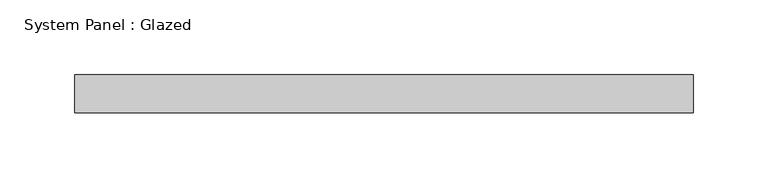
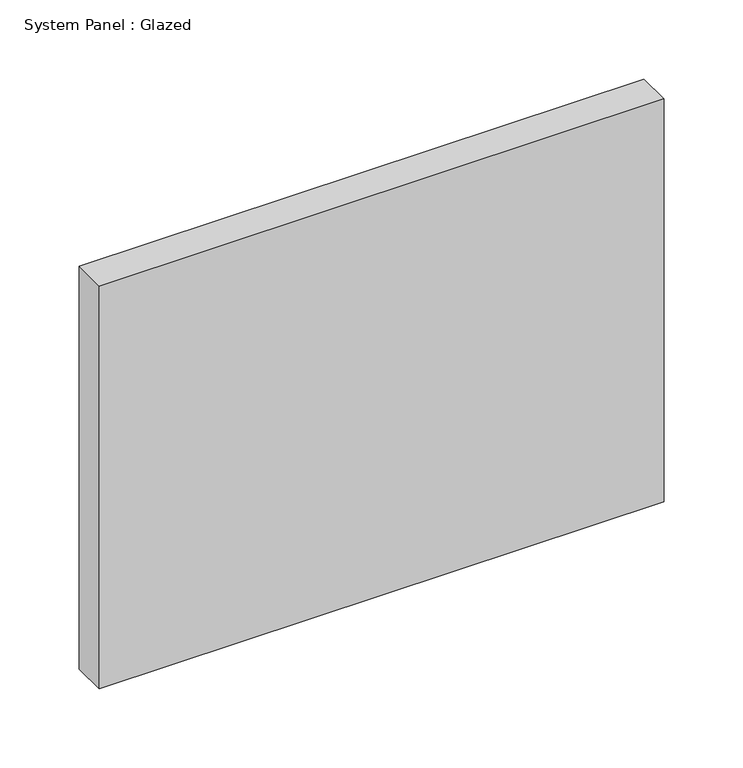
"""IFC4 building model written with IfcOpenShell, lengths in millimetres: plate geometry, System Panel : Glazed."""

from ifc_helpers import new_model, si_unit, origin, origin_with_axes, place, context, project, spatial, polyline, outline, extrude, source, transform, mapped, element, save


def system_panel_glazed_534e268b(model_context):
    return source(origin(), model_context, "Body", "SweptSolid", [
        extrude(outline(polyline([(206.375, 19.05), (-206.375, 19.05), (-206.375, 44.45), (206.375, 44.45), (206.375, 19.05)])), origin_with_axes(), (0.0, 0.0, 1.0), 311.15),
    ])


if __name__ == "__main__":
    model = new_model("IFC4")
    model_context = context("Model", 3, world=origin())
    ifc_project = project(units=[si_unit("LENGTHUNIT", "METRE", prefix="MILLI")], contexts=[model_context])
    site = spatial("IfcSite", under=ifc_project)
    building = spatial("IfcBuilding", under=site)
    placement = place(None, origin())
    system_panel_glazed_shape = system_panel_glazed_534e268b(model_context)
    element("IfcPlate", 1, ObjectType="System Panel : Glazed", at=placement, inside=building, context=model_context, shape_type="MappedRepresentation", body=[
        mapped(system_panel_glazed_shape, transform((0.0, 0.0, 0.0), x_axis=(1.0, 0.0, 0.0), y_axis=(0.0, 1.0, 0.0), z_axis=(0.0, 0.0, 1.0))),
    ])
    save(model, "model.ifc")

# Revit data of these elements
# Type "System Panel : Glazed"
#   Construction Type Id = "GSP4R"
#   Analytic Construction = "1/8 in Pilkington single glazing"
#   Visual Light Transmittance = 0.9
#   Solar Heat Gain Coefficient = 0.86
#   Heat Transfer Coefficient (U) = 1.18115 BTU/(h·ft²·°F)
#   Define Thermal Properties by = 1
# Element 1 (IfcPlate, "System Panel : Glazed")
#   Materials on its faces: "Glass"
# Materials
#   "Glass": class "Glass", colour RGB 0 128 192, transparency 0.75, Description = "Soda Lime Glass", Cost = 0
